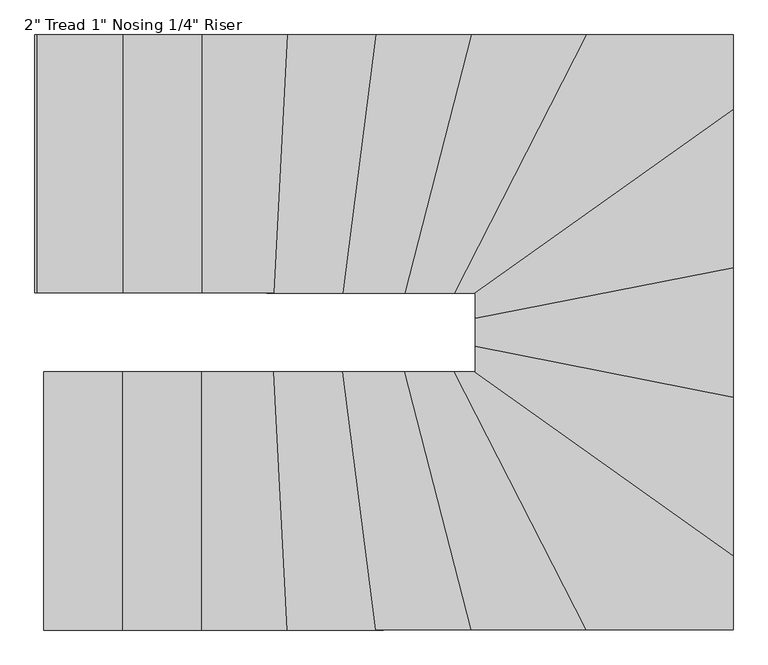
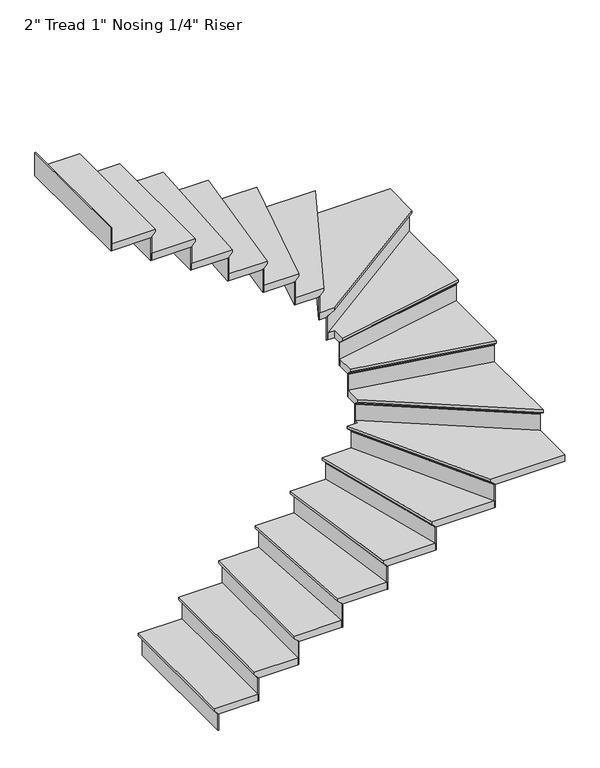
"""IFC4 building model written with IfcOpenShell, lengths in millimetres: stair flight geometry."""

from ifc_helpers import new_model, si_unit, origin, place, context, project, spatial, faceted_brep, source, transform, mapped, element, save


def stair_flight_5209112f(model_context):
    return source(origin(), model_context, "Body", "Brep", [
        faceted_brep([(531.7538115, -7565.2090409, 9751.4833333), (531.7538115, -7565.2090409, 9770.5333333), (531.7538115, -6650.8090409, 9770.5333333), (531.7538115, -6650.8090409, 9751.4833333), (557.1538115, -7565.2090409, 9726.0833333), (557.1538115, -6650.8090409, 9726.0833333), (836.5538115, -7565.2090409, 9770.5333333), (836.5538115, -6650.8090409, 9770.5333333), (557.1538115, -6650.8090409, 9719.7333333), (836.5538115, -6650.8090409, 9719.7333333), (836.5538115, -7565.2090409, 9719.7333333), (557.1538115, -7565.2090409, 9719.7333333)], [[[0, 1, 2, 3]], [[4, 0, 3, 5]], [[2, 1, 6, 7]], [[8, 9, 10, 11]], [[2, 7, 9, 8, 5, 3]], [[8, 11, 4, 5]], [[6, 1, 0, 4, 11, 10]], [[7, 6, 10, 9]]]),
        faceted_brep([(557.1538115, -7565.2090409, 9719.7333333), (557.1538115, -7565.2090409, 9601.2), (563.5038115, -7565.2090409, 9601.2), (563.5038115, -7565.2090409, 9719.7333333), (557.1538115, -6650.8090409, 9719.7333333), (563.5038115, -6650.8090409, 9719.7333333), (563.5038115, -6650.8090409, 9601.2), (557.1538115, -6650.8090409, 9601.2)], [[[0, 1, 2, 3]], [[4, 5, 6, 7]], [[1, 0, 4, 7]], [[2, 1, 7, 6]], [[3, 2, 6, 5]], [[0, 3, 5, 4]]]),
        faceted_brep([(836.5538115, -7565.2090409, 9889.0666667), (836.5538115, -7565.2090409, 9719.7333333), (842.9038115, -7565.2090409, 9719.7333333), (842.9038115, -7565.2090409, 9889.0666667), (836.5538115, -6650.8090409, 9889.0666667), (842.9038115, -6650.8090409, 9889.0666667), (842.9038115, -6650.8090409, 9719.7333333), (836.5538115, -6650.8090409, 9719.7333333)], [[[0, 1, 2, 3]], [[4, 5, 6, 7]], [[1, 0, 4, 7]], [[2, 1, 7, 6]], [[3, 2, 6, 5]], [[0, 3, 5, 4]]]),
        faceted_brep([(811.1538115, -6650.8090409, 9939.8666667), (811.1538115, -7565.2090409, 9939.8666667), (1115.9538115, -7565.2090409, 9939.8666667), (1115.9538115, -6650.8090409, 9939.8666667), (836.5538115, -6650.8090409, 9889.0666667), (1115.9538115, -6650.8090409, 9889.0666667), (1115.9538115, -7565.2090409, 9889.0666667), (836.5538115, -7565.2090409, 9889.0666667), (836.5538115, -6650.8090409, 9895.4166667), (811.1538115, -6650.8090409, 9920.8166667), (836.5538115, -7565.2090409, 9895.4166667), (811.1538115, -7565.2090409, 9920.8166667)], [[[0, 1, 2, 3]], [[4, 5, 6, 7]], [[0, 3, 5, 4, 8, 9]], [[4, 7, 10, 8]], [[2, 1, 11, 10, 7, 6]], [[3, 2, 6, 5]], [[11, 1, 0, 9]], [[10, 11, 9, 8]]]),
        faceted_brep([(1115.9538115, -7565.2090409, 10058.4), (1115.9538115, -7565.2090409, 9889.0666667), (1122.3038115, -7565.2090409, 9889.0666667), (1122.3038115, -7565.2090409, 10058.4), (1115.9538115, -6650.8090409, 10058.4), (1122.3038115, -6650.8090409, 10058.4), (1122.3038115, -6650.8090409, 9889.0666667), (1115.9538115, -6650.8090409, 9889.0666667)], [[[0, 1, 2, 3]], [[4, 5, 6, 7]], [[1, 0, 4, 7]], [[2, 1, 7, 6]], [[3, 2, 6, 5]], [[0, 3, 5, 4]]]),
        faceted_brep([(1090.5538115, -6650.8090409, 10109.2), (1090.5538115, -7565.2090409, 10109.2), (1419.1552434, -7565.2090409, 10109.2), (1371.620973, -6650.8090409, 10109.2), (1115.9538115, -6650.8090409, 10058.4), (1371.620973, -6650.8090409, 10058.4), (1419.1552434, -7565.2090409, 10058.4), (1115.9538115, -7565.2090409, 10058.4), (1115.9538115, -6650.8090409, 10064.75), (1090.5538115, -6650.8090409, 10090.15), (1115.9538115, -7565.2090409, 10064.75), (1090.5538115, -7565.2090409, 10090.15)], [[[0, 1, 2, 3]], [[4, 5, 6, 7]], [[0, 3, 5, 4, 8, 9]], [[4, 7, 10, 8]], [[2, 1, 11, 10, 7, 6]], [[3, 2, 6, 5]], [[11, 1, 0, 9]], [[10, 11, 9, 8]]]),
        faceted_brep([(1419.1552434, -7565.2090409, 10227.7333333), (1419.1552434, -7565.2090409, 10058.4), (1425.5138176, -7565.2090409, 10058.4), (1425.5138176, -7565.2090409, 10227.7333333), (1371.620973, -6650.8090409, 10227.7333333), (1377.9795471, -6650.8090409, 10227.7333333), (1377.9795471, -6650.8090409, 10058.4), (1371.620973, -6650.8090409, 10058.4)], [[[0, 1, 2, 3]], [[4, 5, 6, 7]], [[1, 0, 4, 7]], [[2, 1, 7, 6]], [[3, 2, 6, 5]], [[0, 3, 5, 4]]]),
        faceted_brep([(1346.1866763, -6650.8090409, 10278.5333333), (1393.7209467, -7565.2090409, 10278.5333333), (1734.1437245, -7565.2090409, 10278.5333333), (1615.7876728, -6650.8090409, 10278.5333333), (1371.620973, -6650.8090409, 10227.7333333), (1615.7876728, -6650.8090409, 10227.7333333), (1734.1437245, -7565.2090409, 10227.7333333), (1419.1552434, -7565.2090409, 10227.7333333), (1371.620973, -6650.8090409, 10234.0833333), (1346.1866763, -6650.8090409, 10259.4833333), (1419.1552434, -7565.2090409, 10234.0833333), (1393.7209467, -7565.2090409, 10259.4833333)], [[[0, 1, 2, 3]], [[4, 5, 6, 7]], [[0, 3, 5, 4, 8, 9]], [[4, 7, 10, 8]], [[2, 1, 11, 10, 7, 6]], [[3, 2, 6, 5]], [[11, 1, 0, 9]], [[10, 11, 9, 8]]]),
        faceted_brep([(1734.1437245, -7565.2090409, 10397.0666667), (1734.1437245, -7565.2090409, 10227.7333333), (1740.5466962, -7565.2090409, 10227.7333333), (1740.5466962, -7565.2090409, 10397.0666667), (1615.7876728, -6650.8090409, 10397.0666667), (1622.1906446, -6650.8090409, 10397.0666667), (1622.1906446, -6650.8090409, 10227.7333333), (1615.7876728, -6650.8090409, 10227.7333333)], [[[0, 1, 2, 3]], [[4, 5, 6, 7]], [[1, 0, 4, 7]], [[2, 1, 7, 6]], [[3, 2, 6, 5]], [[0, 3, 5, 4]]]),
        faceted_brep([(1590.1757857, -6650.8090409, 10447.8666667), (1708.5318374, -7565.2090409, 10447.8666667), (2072.5453427, -7565.2090409, 10447.8666667), (1837.4148953, -6650.8090409, 10447.8666667), (1615.7876728, -6650.8090409, 10397.0666667), (1837.4148953, -6650.8090409, 10397.0666667), (2072.5453427, -7565.2090409, 10397.0666667), (1734.1437245, -7565.2090409, 10397.0666667), (1615.7876728, -6650.8090409, 10403.4166667), (1590.1757857, -6650.8090409, 10428.8166667), (1734.1437245, -7565.2090409, 10403.4166667), (1708.5318374, -7565.2090409, 10428.8166667)], [[[0, 1, 2, 3]], [[4, 5, 6, 7]], [[0, 3, 5, 4, 8, 9]], [[4, 7, 10, 8]], [[2, 1, 11, 10, 7, 6]], [[3, 2, 6, 5]], [[11, 1, 0, 9]], [[10, 11, 9, 8]]]),
        faceted_brep([(2072.5453427, -7565.2090409, 10566.4), (2072.5453427, -7565.2090409, 10397.0666667), (2079.1019196, -7565.2090409, 10397.0666667), (2079.1019196, -7565.2090409, 10566.4), (1837.4148953, -6650.8090409, 10566.4), (1843.9714722, -6650.8090409, 10566.4), (1843.9714722, -6650.8090409, 10397.0666667), (1837.4148953, -6650.8090409, 10397.0666667)], [[[0, 1, 2, 3]], [[4, 5, 6, 7]], [[1, 0, 4, 7]], [[2, 1, 7, 6]], [[3, 2, 6, 5]], [[0, 3, 5, 4]]]),
        faceted_brep([(1811.1885878, -6650.8090409, 10617.2), (2046.3190352, -7565.2090409, 10617.2), (2482.5861527, -7565.2090409, 10617.2), (2013.7615314, -6650.8090409, 10617.2), (1837.4148953, -6650.8090409, 10566.4), (2013.7615314, -6650.8090409, 10566.4), (2482.5861527, -7565.2090409, 10566.4), (2072.5453427, -7565.2090409, 10566.4), (1837.4148953, -6650.8090409, 10572.75), (1811.1885878, -6650.8090409, 10598.15), (2072.5453427, -7565.2090409, 10572.75), (2046.3190352, -7565.2090409, 10598.15)], [[[0, 1, 2, 3]], [[4, 5, 6, 7]], [[0, 3, 5, 4, 8, 9]], [[4, 7, 10, 8]], [[2, 1, 11, 10, 7, 6]], [[3, 2, 6, 5]], [[11, 1, 0, 9]], [[10, 11, 9, 8]]]),
        faceted_brep([(2482.5861527, -7565.2090409, 10735.7333333), (2482.5861527, -7565.2090409, 10566.4), (2489.7221358, -7565.2090409, 10566.4), (2489.7221358, -7565.2090409, 10735.7333333), (2013.7615314, -6650.8090409, 10735.7333333), (2020.8975145, -6650.8090409, 10735.7333333), (2020.8975145, -6650.8090409, 10566.4), (2013.7615314, -6650.8090409, 10566.4)], [[[0, 1, 2, 3]], [[4, 5, 6, 7]], [[1, 0, 4, 7]], [[2, 1, 7, 6]], [[3, 2, 6, 5]], [[0, 3, 5, 4]]]),
        faceted_brep([(2059.4855034, -6621.253958, 10786.5333333), (2059.4855034, -6650.8090409, 10786.5333333), (1985.2175988, -6650.8090409, 10786.5333333), (2454.0422202, -7565.2090409, 10786.5333333), (2973.8855034, -7565.2090409, 10786.5333333), (2973.8855034, -7271.5279072, 10786.5333333), (2059.4855034, -6650.8090409, 10735.7333333), (2059.4855034, -6621.253958, 10735.7333333), (2973.8855034, -7271.5279072, 10735.7333333), (2973.8855034, -7565.2090409, 10735.7333333), (2482.5861527, -7565.2090409, 10735.7333333), (2013.7615314, -6650.8090409, 10735.7333333), (2013.7615314, -6650.8090409, 10742.0833333), (1985.2175988, -6650.8090409, 10767.4833333), (2482.5861527, -7565.2090409, 10742.0833333), (2454.0422202, -7565.2090409, 10767.4833333)], [[[0, 1, 2, 3, 4, 5]], [[6, 7, 8, 9, 10, 11]], [[1, 0, 7, 6]], [[2, 1, 6, 11, 12, 13]], [[11, 10, 14, 12]], [[4, 3, 15, 14, 10, 9]], [[5, 4, 9, 8]], [[0, 5, 8, 7]], [[15, 3, 2, 13]], [[14, 15, 13, 12]]]),
        faceted_brep([(2973.8855034, -7271.5279072, 10905.0666667), (2973.8855034, -7271.5279072, 10735.7333333), (2973.8855034, -7263.7359324, 10735.7333333), (2973.8855034, -7263.7359324, 10905.0666667), (2059.4855034, -6621.253958, 10905.0666667), (2059.4855034, -6613.4619832, 10905.0666667), (2059.4855034, -6613.4619832, 10735.7333333), (2059.4855034, -6621.253958, 10735.7333333)], [[[0, 1, 2, 3]], [[4, 5, 6, 7]], [[1, 0, 4, 7]], [[2, 1, 7, 6]], [[3, 2, 6, 5]], [[0, 3, 5, 4]]]),
        faceted_brep([(2059.4855034, -6652.4218572, 10955.8666667), (2973.8855034, -7302.6958063, 10955.8666667), (2973.8855034, -6715.0407273, 10955.8666667), (2059.4855034, -6534.7998709, 10955.8666667), (2059.4855034, -6621.253958, 10905.0666667), (2059.4855034, -6534.7998709, 10905.0666667), (2973.8855034, -6715.0407273, 10905.0666667), (2973.8855034, -7271.5279072, 10905.0666667), (2059.4855034, -6621.253958, 10911.4166667), (2059.4855034, -6652.4218572, 10936.8166667), (2973.8855034, -7271.5279072, 10911.4166667), (2973.8855034, -7302.6958063, 10936.8166667)], [[[0, 1, 2, 3]], [[4, 5, 6, 7]], [[0, 3, 5, 4, 8, 9]], [[4, 7, 10, 8]], [[3, 2, 6, 5]], [[11, 1, 0, 9]], [[10, 11, 9, 8]], [[2, 1, 11, 10, 7, 6]]]),
        faceted_brep([(2973.8855034, -6715.0407273, 11074.4), (2973.8855034, -6715.0407273, 10905.0666667), (2973.8855034, -6708.5685418, 10905.0666667), (2973.8855034, -6708.5685418, 11074.4), (2059.4855034, -6534.7998709, 11074.4), (2059.4855034, -6528.3276855, 11074.4), (2059.4855034, -6528.3276855, 10905.0666667), (2059.4855034, -6534.7998709, 10905.0666667)], [[[0, 1, 2, 3]], [[4, 5, 6, 7]], [[1, 0, 4, 7]], [[2, 1, 7, 6]], [[3, 2, 6, 5]], [[0, 3, 5, 4]]]),
        faceted_brep([(2059.4855034, -6560.6886127, 11125.2), (2973.8855034, -6740.929469, 11125.2), (2973.8855034, -6255.3998709, 11125.2), (2059.4855034, -6435.6407273, 11125.2), (2059.4855034, -6534.7998709, 11074.4), (2059.4855034, -6435.6407273, 11074.4), (2973.8855034, -6255.3998709, 11074.4), (2973.8855034, -6715.0407273, 11074.4), (2059.4855034, -6534.7998709, 11080.75), (2059.4855034, -6560.6886127, 11106.15), (2973.8855034, -6715.0407273, 11080.75), (2973.8855034, -6740.929469, 11106.15)], [[[0, 1, 2, 3]], [[4, 5, 6, 7]], [[0, 3, 5, 4, 8, 9]], [[4, 7, 10, 8]], [[2, 1, 11, 10, 7, 6]], [[3, 2, 6, 5]], [[11, 1, 0, 9]], [[10, 11, 9, 8]]]),
        faceted_brep([(2973.8855034, -6255.3998709, 11243.7333333), (2973.8855034, -6255.3998709, 11074.4), (2973.8855034, -6248.9276855, 11074.4), (2973.8855034, -6248.9276855, 11243.7333333), (2059.4855034, -6435.6407273, 11243.7333333), (2059.4855034, -6429.1685418, 11243.7333333), (2059.4855034, -6429.1685418, 11074.4), (2059.4855034, -6435.6407273, 11074.4)], [[[0, 1, 2, 3]], [[4, 5, 6, 7]], [[1, 0, 4, 7]], [[2, 1, 7, 6]], [[3, 2, 6, 5]], [[0, 3, 5, 4]]]),
        faceted_brep([(2013.3900289, -6371.4090409, 11294.5333333), (2059.4855034, -6371.4090409, 11294.5333333), (2059.4855034, -6461.529469, 11294.5333333), (2973.8855034, -6281.2886127, 11294.5333333), (2973.8855034, -5688.3543762, 11294.5333333), (2059.4855034, -6371.4090409, 11243.7333333), (2013.3900289, -6371.4090409, 11243.7333333), (2973.8855034, -5688.3543762, 11243.7333333), (2973.8855034, -6255.3998709, 11243.7333333), (2059.4855034, -6435.6407273, 11243.7333333), (2973.8855034, -6255.3998709, 11250.0833333), (2059.4855034, -6435.6407273, 11250.0833333), (2973.8855034, -6281.2886127, 11275.4833333), (2059.4855034, -6461.529469, 11275.4833333)], [[[0, 1, 2, 3, 4]], [[5, 6, 7, 8, 9]], [[1, 0, 6, 5]], [[9, 8, 10, 11]], [[4, 3, 12, 10, 8, 7]], [[0, 4, 7, 6]], [[12, 3, 2, 13]], [[10, 12, 13, 11]], [[2, 1, 5, 9, 11, 13]]]),
        faceted_brep([(2973.8855034, -5688.3543762, 11413.0666667), (2973.8855034, -5688.3543762, 11243.7333333), (2973.8855034, -5680.5624014, 11243.7333333), (2973.8855034, -5680.5624014, 11413.0666667), (2013.3900289, -6371.4090409, 11413.0666667), (2002.4331364, -6371.4090409, 11413.0666667), (2002.4331364, -6371.4090409, 11243.7333333), (2013.3900289, -6371.4090409, 11243.7333333)], [[[0, 1, 2, 3]], [[4, 5, 6, 7]], [[1, 0, 4, 7]], [[2, 1, 7, 6]], [[3, 2, 6, 5]], [[0, 3, 5, 4]]]),
        faceted_brep([(2057.2175988, -6371.4090409, 11463.8666667), (2973.8855034, -5719.5222754, 11463.8666667), (2973.8855034, -5457.0090409, 11463.8666667), (2425.4982876, -5457.0090409, 11463.8666667), (1956.6736663, -6371.4090409, 11463.8666667), (2013.3900289, -6371.4090409, 11413.0666667), (1956.6736663, -6371.4090409, 11413.0666667), (2425.4982876, -5457.0090409, 11413.0666667), (2973.8855034, -5457.0090409, 11413.0666667), (2973.8855034, -5688.3543762, 11413.0666667), (2013.3900289, -6371.4090409, 11419.4166667), (2057.2175988, -6371.4090409, 11444.8166667), (2973.8855034, -5688.3543762, 11419.4166667), (2973.8855034, -5719.5222754, 11444.8166667)], [[[0, 1, 2, 3, 4]], [[5, 6, 7, 8, 9]], [[0, 4, 6, 5, 10, 11]], [[5, 9, 12, 10]], [[2, 1, 13, 12, 9, 8]], [[4, 3, 7, 6]], [[13, 1, 0, 11]], [[12, 13, 11, 10]], [[3, 2, 8, 7]]]),
        faceted_brep([(2425.4982876, -5457.0090409, 11582.4), (2425.4982876, -5457.0090409, 11413.0666667), (2418.3623045, -5457.0090409, 11413.0666667), (2418.3623045, -5457.0090409, 11582.4), (1956.6736663, -6371.4090409, 11582.4), (1949.5376832, -6371.4090409, 11582.4), (1949.5376832, -6371.4090409, 11413.0666667), (1956.6736663, -6371.4090409, 11413.0666667)], [[[0, 1, 2, 3]], [[4, 5, 6, 7]], [[1, 0, 4, 7]], [[2, 1, 7, 6]], [[3, 2, 6, 5]], [[0, 3, 5, 4]]]),
        faceted_brep([(1985.2175988, -6371.4090409, 11633.2), (2454.0422202, -5457.0090409, 11633.2), (2020.0927278, -5457.0090409, 11633.2), (1784.9622804, -6371.4090409, 11633.2), (1956.6736663, -6371.4090409, 11582.4), (1784.9622804, -6371.4090409, 11582.4), (2020.0927278, -5457.0090409, 11582.4), (2425.4982876, -5457.0090409, 11582.4), (1956.6736663, -6371.4090409, 11588.75), (1985.2175988, -6371.4090409, 11614.15), (2425.4982876, -5457.0090409, 11588.75), (2454.0422202, -5457.0090409, 11614.15)], [[[0, 1, 2, 3]], [[4, 5, 6, 7]], [[0, 3, 5, 4, 8, 9]], [[4, 7, 10, 8]], [[2, 1, 11, 10, 7, 6]], [[3, 2, 6, 5]], [[11, 1, 0, 9]], [[10, 11, 9, 8]]]),
        faceted_brep([(2020.0927278, -5457.0090409, 11751.7333333), (2020.0927278, -5457.0090409, 11582.4), (2013.5361509, -5457.0090409, 11582.4), (2013.5361509, -5457.0090409, 11751.7333333), (1784.9622804, -6371.4090409, 11751.7333333), (1778.4057035, -6371.4090409, 11751.7333333), (1778.4057035, -6371.4090409, 11582.4), (1784.9622804, -6371.4090409, 11582.4)], [[[0, 1, 2, 3]], [[4, 5, 6, 7]], [[1, 0, 4, 7]], [[2, 1, 7, 6]], [[3, 2, 6, 5]], [[0, 3, 5, 4]]]),
        faceted_brep([(1811.1885878, -6371.4090409, 11802.5333333), (2046.3190352, -5457.0090409, 11802.5333333), (1682.9199502, -5457.0090409, 11802.5333333), (1564.5638986, -6371.4090409, 11802.5333333), (1784.9622804, -6371.4090409, 11751.7333333), (1564.5638986, -6371.4090409, 11751.7333333), (1682.9199502, -5457.0090409, 11751.7333333), (2020.0927278, -5457.0090409, 11751.7333333), (1784.9622804, -6371.4090409, 11758.0833333), (1811.1885878, -6371.4090409, 11783.4833333), (2020.0927278, -5457.0090409, 11758.0833333), (2046.3190352, -5457.0090409, 11783.4833333)], [[[0, 1, 2, 3]], [[4, 5, 6, 7]], [[0, 3, 5, 4, 8, 9]], [[4, 7, 10, 8]], [[2, 1, 11, 10, 7, 6]], [[3, 2, 6, 5]], [[11, 1, 0, 9]], [[10, 11, 9, 8]]]),
        faceted_brep([(1682.9199502, -5457.0090409, 11921.0666667), (1682.9199502, -5457.0090409, 11751.7333333), (1676.5169785, -5457.0090409, 11751.7333333), (1676.5169785, -5457.0090409, 11921.0666667), (1564.5638986, -6371.4090409, 11921.0666667), (1558.1609268, -6371.4090409, 11921.0666667), (1558.1609268, -6371.4090409, 11751.7333333), (1564.5638986, -6371.4090409, 11751.7333333)], [[[0, 1, 2, 3]], [[4, 5, 6, 7]], [[1, 0, 4, 7]], [[2, 1, 7, 6]], [[3, 2, 6, 5]], [[0, 3, 5, 4]]]),
        faceted_brep([(1590.1757857, -6371.4090409, 11971.8666667), (1708.5318374, -5457.0090409, 11971.8666667), (1368.2866501, -5457.0090409, 11971.8666667), (1320.7523797, -6371.4090409, 11971.8666667), (1564.5638986, -6371.4090409, 11921.0666667), (1320.7523797, -6371.4090409, 11921.0666667), (1368.2866501, -5457.0090409, 11921.0666667), (1682.9199502, -5457.0090409, 11921.0666667), (1564.5638986, -6371.4090409, 11927.4166667), (1590.1757857, -6371.4090409, 11952.8166667), (1682.9199502, -5457.0090409, 11927.4166667), (1708.5318374, -5457.0090409, 11952.8166667)], [[[0, 1, 2, 3]], [[4, 5, 6, 7]], [[0, 3, 5, 4, 8, 9]], [[4, 7, 10, 8]], [[2, 1, 11, 10, 7, 6]], [[3, 2, 6, 5]], [[11, 1, 0, 9]], [[10, 11, 9, 8]]]),
        faceted_brep([(1368.2866501, -5457.0090409, 12090.4), (1368.2866501, -5457.0090409, 11921.0666667), (1361.9280759, -5457.0090409, 11921.0666667), (1361.9280759, -5457.0090409, 12090.4), (1320.7523797, -6371.4090409, 12090.4), (1314.3938055, -6371.4090409, 12090.4), (1314.3938055, -6371.4090409, 11921.0666667), (1320.7523797, -6371.4090409, 11921.0666667)], [[[0, 1, 2, 3]], [[4, 5, 6, 7]], [[1, 0, 4, 7]], [[2, 1, 7, 6]], [[3, 2, 6, 5]], [[0, 3, 5, 4]]]),
        faceted_brep([(1346.1866763, -6371.4090409, 12141.2), (1393.7209467, -5457.0090409, 12141.2), (1065.1538115, -5457.0090409, 12141.2), (1065.1538115, -6371.4090409, 12141.2), (1320.7523797, -6371.4090409, 12090.4), (1065.1538115, -6371.4090409, 12090.4), (1065.1538115, -5457.0090409, 12090.4), (1368.2866501, -5457.0090409, 12090.4), (1320.7523797, -6371.4090409, 12096.75), (1346.1866763, -6371.4090409, 12122.15), (1368.2866501, -5457.0090409, 12096.75), (1393.7209467, -5457.0090409, 12122.15)], [[[0, 1, 2, 3]], [[4, 5, 6, 7]], [[0, 3, 5, 4, 8, 9]], [[4, 7, 10, 8]], [[2, 1, 11, 10, 7, 6]], [[3, 2, 6, 5]], [[11, 1, 0, 9]], [[10, 11, 9, 8]]]),
        faceted_brep([(1065.1538115, -5457.0090409, 12259.7333333), (1065.1538115, -5457.0090409, 12090.4), (1058.8038115, -5457.0090409, 12090.4), (1058.8038115, -5457.0090409, 12259.7333333), (1065.1538115, -6371.4090409, 12259.7333333), (1058.8038115, -6371.4090409, 12259.7333333), (1058.8038115, -6371.4090409, 12090.4), (1065.1538115, -6371.4090409, 12090.4)], [[[0, 1, 2, 3]], [[4, 5, 6, 7]], [[1, 0, 4, 7]], [[2, 1, 7, 6]], [[3, 2, 6, 5]], [[0, 3, 5, 4]]]),
        faceted_brep([(1090.5538115, -6371.4090409, 12310.5333333), (1090.5538115, -5457.0090409, 12310.5333333), (785.7538115, -5457.0090409, 12310.5333333), (785.7538115, -6371.4090409, 12310.5333333), (1065.1538115, -6371.4090409, 12259.7333333), (785.7538115, -6371.4090409, 12259.7333333), (785.7538115, -5457.0090409, 12259.7333333), (1065.1538115, -5457.0090409, 12259.7333333), (1065.1538115, -6371.4090409, 12266.0833333), (1090.5538115, -6371.4090409, 12291.4833333), (1065.1538115, -5457.0090409, 12266.0833333), (1090.5538115, -5457.0090409, 12291.4833333)], [[[0, 1, 2, 3]], [[4, 5, 6, 7]], [[0, 3, 5, 4, 8, 9]], [[4, 7, 10, 8]], [[2, 1, 11, 10, 7, 6]], [[3, 2, 6, 5]], [[11, 1, 0, 9]], [[10, 11, 9, 8]]]),
        faceted_brep([(785.7538115, -5457.0090409, 12429.0666667), (785.7538115, -5457.0090409, 12259.7333333), (779.4038115, -5457.0090409, 12259.7333333), (779.4038115, -5457.0090409, 12429.0666667), (785.7538115, -6371.4090409, 12429.0666667), (779.4038115, -6371.4090409, 12429.0666667), (779.4038115, -6371.4090409, 12259.7333333), (785.7538115, -6371.4090409, 12259.7333333)], [[[0, 1, 2, 3]], [[4, 5, 6, 7]], [[1, 0, 4, 7]], [[2, 1, 7, 6]], [[3, 2, 6, 5]], [[0, 3, 5, 4]]]),
        faceted_brep([(506.3538115, -5457.0090409, 12598.4), (506.3538115, -5457.0090409, 12429.0666667), (500.0038115, -5457.0090409, 12429.0666667), (500.0038115, -5457.0090409, 12598.4), (506.3538115, -6371.4090409, 12598.4), (500.0038115, -6371.4090409, 12598.4), (500.0038115, -6371.4090409, 12429.0666667), (506.3538115, -6371.4090409, 12429.0666667)], [[[0, 1, 2, 3]], [[4, 5, 6, 7]], [[1, 0, 4, 7]], [[2, 1, 7, 6]], [[3, 2, 6, 5]], [[0, 3, 5, 4]]]),
        faceted_brep([(811.1538115, -6371.4090409, 12479.8666667), (811.1538115, -5457.0090409, 12479.8666667), (506.3538115, -5457.0090409, 12479.8666667), (506.3538115, -6371.4090409, 12479.8666667), (785.7538115, -6371.4090409, 12429.0666667), (506.3538115, -6371.4090409, 12429.0666667), (506.3538115, -5457.0090409, 12429.0666667), (785.7538115, -5457.0090409, 12429.0666667), (785.7538115, -6371.4090409, 12435.4166667), (811.1538115, -6371.4090409, 12460.8166667), (785.7538115, -5457.0090409, 12435.4166667), (811.1538115, -5457.0090409, 12460.8166667)], [[[0, 1, 2, 3]], [[4, 5, 6, 7]], [[0, 3, 5, 4, 8, 9]], [[4, 7, 10, 8]], [[2, 1, 11, 10, 7, 6]], [[3, 2, 6, 5]], [[11, 1, 0, 9]], [[10, 11, 9, 8]]]),
    ])


if __name__ == "__main__":
    model = new_model("IFC4")
    model_context = context("Model", 3, world=origin())
    ifc_project = project(units=[si_unit("LENGTHUNIT", "METRE", prefix="MILLI")], contexts=[model_context])
    site = spatial("IfcSite", under=ifc_project)
    building = spatial("IfcBuilding", under=site)
    placement = place(None, origin())
    stair_flight_shape = stair_flight_5209112f(model_context)
    element("IfcStairFlight", 1, ObjectType="2\" Tread 1\" Nosing 1/4\" Riser", at=placement, inside=building, context=model_context, shape_type="MappedRepresentation", body=[
        mapped(stair_flight_shape, transform((0.0, 0.0, 0.0), x_axis=(1.0, 0.0, 0.0), y_axis=(0.0, 1.0, 0.0), z_axis=(0.0, 0.0, 1.0))),
    ])
    save(model, "model.ifc")
